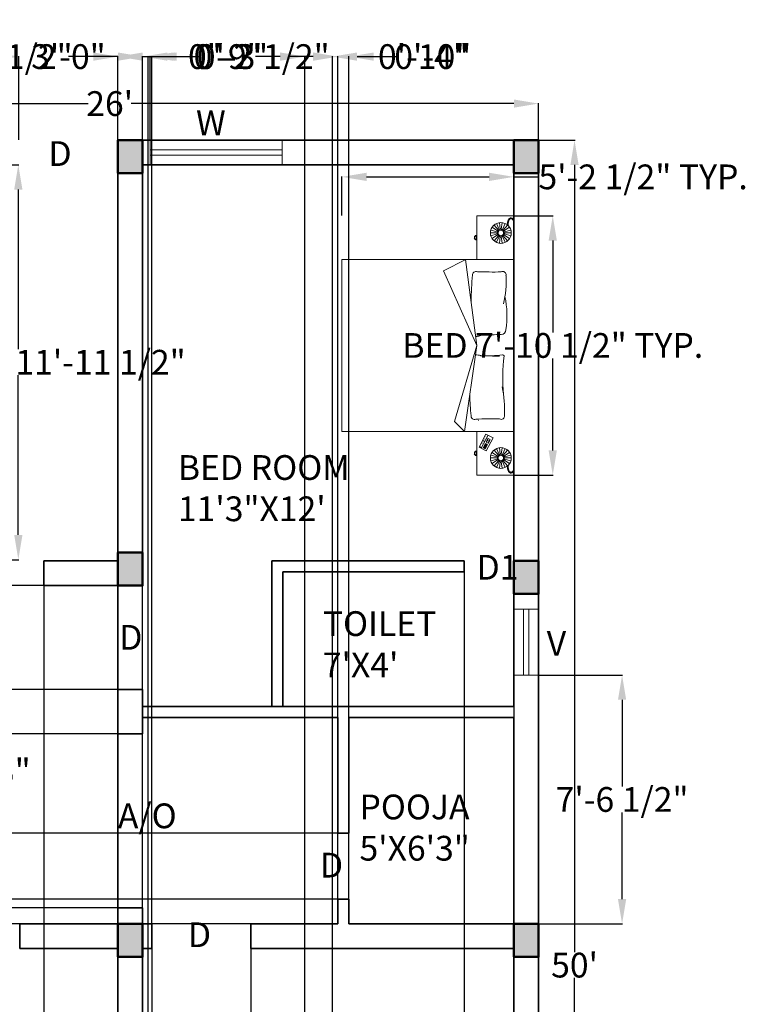
# Model space of a CAD drawing. Units: inches. Extents: x 113 to 575, y 111 to 799.
# Tile 4 of 4: x 301 to 565, y 441 to 799. Entities that reach past the tile are written whole.
import ezdxf

# ---------------------------------------------------------------- set-up
doc = ezdxf.new("R2010")
doc.units = ezdxf.units.IN
doc.header["$MEASUREMENT"] = 0
for name, color, linetype, lineweight in [('A-ANNO-DIMS', 2, 'Continuous', 18), ('A-ANNO-TEXT', 7, 'Continuous', 18), ('A-AREA-IDEN', 7, 'Continuous', 25), ('A-COLS', 7, 'Continuous', 50), ('A-COLS-PATT', 252, 'Continuous', 13), ('A-FURN', 8, 'Continuous', 18), ('A-GLAZ', 4, 'Continuous', 18), ('A-WALL', 7, 'Continuous', 35)]:
    doc.layers.add(name, color=color, linetype=linetype, lineweight=lineweight)
doc.styles.get("Standard").update_dxf_attribs({"font": 'arial.ttf'})
doc.dimstyles.get("Standard").update_dxf_attribs({"dimtxt": 9, "dimasz": 9, "dimexe": 0.18, "dimexo": 0.0625, "dimgap": 0.09, "dimtad": 0, "dimtih": 1, "dimtoh": 1, "dimdec": 0, "dimzin": 0, "dimdsep": 46, "dimlunit": 3, "dimtxsty": 'Standard', "dimcen": 0.09, "dimadec": 0, "dimazin": 0, "dimtfac": 1, "dimtdec": 0, "dimtofl": 0, "dimtmove": 0, "dimatfit": 3, "dimfxl": 1, "dimtolj": 1, "dimtzin": 0, "dimarcsym": 0})

# ---------------------------------------------------------------- blocks, each defined once
blk = doc.blocks.new('23')
for p, q in [((198.051, 218.551), (197.59, 218.551)), ((197.59, 218.551), (197.59, 218.161)), ((198.051, 218.551), (197.59, 218.551)), ((197.688, 218.484), (197.741, 218.439)), ((197.711, 218.505), (197.749, 218.446)), ((197.74, 218.518), (197.76, 218.451)), ((197.771, 218.522), (197.771, 218.452)), ((197.771, 218.522), (197.771, 218.452)), ((197.802, 218.518), (197.782, 218.451)), ((197.792, 218.446), (197.83, 218.505)), ((197.801, 218.439), (197.854, 218.484)), ((198.051, 216.732), (198.051, 218.551)), ((198.051, 218.551), (198.96, 218.551)), ((198.051, 218.551), (199.869, 218.551)), ((198.051, 218.551), (198.051, 218.161)), ((199.869, 218.551), (200.331, 218.551)), ((199.869, 218.551), (200.331, 218.551)), ((199.869, 218.551), (199.869, 216.732)), ((200.12, 218.439), (200.067, 218.484)), ((200.129, 218.446), (200.091, 218.505)), ((200.119, 218.518), (200.139, 218.451)), ((200.15, 218.522), (200.15, 218.452)), ((200.15, 218.522), (200.15, 218.452)), ((200.181, 218.518), (200.161, 218.451)), ((200.209, 218.505), (200.171, 218.446)), ((200.233, 218.484), (200.18, 218.439)), ((200.331, 218.551), (200.331, 218.161)), ((197.662, 218.428), (197.731, 218.418)), ((197.662, 218.397), (197.731, 218.407)), ((197.671, 218.458), (197.735, 218.429)), ((197.671, 218.367), (197.735, 218.396)), ((197.688, 218.341), (197.741, 218.387)), ((197.711, 218.32), (197.749, 218.379)), ((197.742, 218.419), (197.732, 218.423)), ((197.744, 218.425), (197.734, 218.427)), ((197.76, 218.375), (197.74, 218.307)), ((197.765, 218.384), (197.765, 218.373)), ((197.772, 218.383), (197.77, 218.373)), ((197.771, 218.373), (197.771, 218.303)), ((197.771, 218.373), (197.771, 218.303)), ((197.782, 218.375), (197.802, 218.307)), ((197.786, 218.438), (197.795, 218.444)), ((197.792, 218.379), (197.83, 218.32)), ((197.793, 218.431), (197.799, 218.44)), ((197.801, 218.387), (197.854, 218.341)), ((197.807, 218.429), (197.87, 218.458)), ((197.807, 218.396), (197.87, 218.367)), ((197.81, 218.418), (197.879, 218.428)), ((197.81, 218.407), (197.879, 218.397)), ((200.111, 218.418), (200.042, 218.428)), ((200.111, 218.407), (200.042, 218.397)), ((200.114, 218.429), (200.05, 218.458)), ((200.114, 218.396), (200.05, 218.367)), ((200.12, 218.387), (200.067, 218.341)), ((200.129, 218.379), (200.091, 218.32)), ((200.139, 218.375), (200.119, 218.307)), ((200.127, 218.431), (200.122, 218.44)), ((200.134, 218.438), (200.125, 218.444)), ((200.149, 218.383), (200.151, 218.373)), ((200.15, 218.373), (200.15, 218.303)), ((200.15, 218.373), (200.15, 218.303)), ((200.155, 218.384), (200.155, 218.373)), ((200.161, 218.375), (200.181, 218.307)), ((200.209, 218.32), (200.171, 218.379)), ((200.177, 218.425), (200.187, 218.427)), ((200.179, 218.419), (200.188, 218.423)), ((200.233, 218.341), (200.18, 218.387)), ((200.25, 218.458), (200.186, 218.429)), ((200.25, 218.367), (200.186, 218.396)), ((200.259, 218.428), (200.189, 218.418)), ((200.259, 218.397), (200.189, 218.407)), ((199.897, 218.255), (199.936, 218.33)), ((199.909, 218.279), (200.047, 218.206)), ((199.936, 218.33), (200.074, 218.257)), ((199.943, 218.278), (199.955, 218.299)), ((199.961, 218.269), (199.943, 218.278)), ((199.955, 218.299), (199.972, 218.29)), ((199.972, 218.29), (199.961, 218.269)), ((199.966, 218.267), (199.977, 218.288)), ((199.983, 218.257), (199.966, 218.267)), ((199.977, 218.288), (199.994, 218.278)), ((199.994, 218.278), (199.983, 218.257)), ((199.997, 218.25), (200.008, 218.271)), ((200.047, 218.235), (200.002, 218.259)), ((200.048, 218.238), (200.003, 218.262)), ((200.05, 218.241), (200.004, 218.265)), ((200.052, 218.245), (200.007, 218.269)), ((200.053, 218.247), (200.008, 218.271)), ((197.592, 218.158), (198.049, 218.158)), ((197.829, 218.158), (197.812, 218.158)), ((197.812, 218.158), (197.812, 218.151)), ((197.829, 218.151), (197.829, 218.158)), ((198.96, 218.158), (198.051, 218.039)), ((198.171, 217.806), (198.96, 218.158)), ((199.763, 217.922), (198.96, 218.158)), ((198.96, 218.158), (199.869, 218.028)), ((200.329, 218.158), (199.872, 218.158)), ((200.034, 218.183), (199.897, 218.255)), ((200.042, 218.226), (199.997, 218.25)), ((200.044, 218.23), (199.999, 218.254)), ((200.046, 218.233), (200, 218.257)), ((200.074, 218.257), (200.034, 218.183)), ((200.053, 218.247), (200.042, 218.226)), ((200.092, 218.151), (200.092, 218.158)), ((200.092, 218.158), (200.108, 218.158)), ((200.108, 218.158), (200.108, 218.151)), ((197.799, 218.149), (197.799, 218.144)), ((197.84, 218.151), (197.801, 218.151)), ((197.801, 218.141), (197.805, 218.141)), ((197.808, 218.139), (197.808, 218.135)), ((197.81, 218.133), (197.831, 218.133)), ((197.833, 218.135), (197.833, 218.141)), ((197.833, 218.141), (197.84, 218.141)), ((197.842, 218.144), (197.842, 218.149)), ((200.078, 218.144), (200.078, 218.149)), ((200.081, 218.151), (200.12, 218.151)), ((200.087, 218.141), (200.081, 218.141)), ((200.087, 218.135), (200.087, 218.141)), ((200.111, 218.133), (200.09, 218.133)), ((200.113, 218.139), (200.113, 218.135)), ((200.12, 218.141), (200.115, 218.141)), ((200.122, 218.149), (200.122, 218.144)), ((198.051, 218.042), (198.171, 217.806)), ((199.869, 218.028), (199.763, 217.922)), ((198.96, 216.732), (198.051, 216.732)), ((198.96, 216.732), (199.869, 216.732))]:
    blk.add_line(p, q)
for centre, radius in [((197.771, 218.413), 0.11), ((200.15, 218.413), 0.11), ((197.771, 218.413), 0.0397), ((197.771, 218.413), 0.0294), ((200.15, 218.413), 0.0397), ((200.15, 218.413), 0.0294)]:
    blk.add_circle(centre, radius)
for centre, radius, start, end in [((198.213, 218.433), 0.035, 78.7278, 211.6095), ((198.213, 218.433), 0.035, 78.7278, 211.6095), ((198.278, 217.379), 1.09, 77.0564, 93.0488), ((198.278, 217.379), 1.09, 77.0564, 93.0488), ((198.648, 217.496), 0.982, 81.4702, 102.1033), ((198.648, 217.496), 0.982, 81.4702, 102.1033), ((198.794, 218.417), 0.0503, 0, 90), ((198.794, 218.417), 0.0503, 0, 90), ((194.58, 218.326), 3.604, 357.4333, 1.4038), ((194.58, 218.326), 3.604, 357.4333, 1.4038), ((192.856, 218.12), 5.995, 0.9126, 2.8341), ((192.856, 218.12), 5.995, 0.9126, 2.8341), ((199.106, 218.403), 0.0559, 128.2265, 148.4948), ((198.082, 218.271), 0.989, 355.8781, 9.3556), ((205.063, 218.104), 5.995, 177.1659, 179.0874), ((199.31, 220.76), 2.326, 264.0962, 274.1102), ((199.106, 218.403), 0.0559, 41.3461, 41.8512), ((199.642, 217.363), 1.09, 86.9512, 102.9436), ((199.642, 217.363), 1.09, 86.9512, 102.9436), ((199.707, 218.417), 0.035, 328.3905, 101.2722), ((199.707, 218.417), 0.035, 328.3905, 101.2722), ((203.34, 218.31), 3.604, 178.5962, 182.5667), ((203.34, 218.31), 3.604, 178.5962, 182.5667), ((197.592, 218.161), 0.0024, 180, 270), ((198.214, 218.15), 0.0362, 156.1084, 279.6576), ((198.214, 218.15), 0.0362, 156.1084, 279.6576), ((198.785, 218.186), 0.0722, 2.6698, 24.3744), ((198.551, 218.114), 0.317, 5.8626, 18.7589), ((199.2, 218.15), 0.14, 159.1632, 182.3748), ((199.134, 218.17), 0.0722, 155.6256, 177.3302), ((199.755, 218.175), 0.00192, 180, 270), ((199.968, 218.228), 0.00141, 90, 270), ((199.968, 218.228), 0.00141, 270, 90), ((199.972, 218.235), 0.00141, 90, 270), ((199.972, 218.235), 0.00141, 270, 90), ((200.031, 218.191), 0.00141, 90, 270), ((200.031, 218.191), 0.00141, 270, 90), ((200.037, 218.2), 0.00141, 90, 270), ((200.037, 218.2), 0.00141, 270, 90), ((200.329, 218.161), 0.0024, 270, 0), ((197.801, 218.149), 0.0024, 90, 180), ((197.801, 218.144), 0.0024, 180, 270), ((197.805, 218.139), 0.0024, 0, 90), ((197.81, 218.135), 0.0024, 180, 270), ((197.831, 218.135), 0.0024, 270, 0), ((197.84, 218.149), 0.0024, 0, 90), ((197.84, 218.144), 0.0024, 270, 0), ((198.502, 220.904), 2.805, 264.1139, 269.9157), ((198.502, 220.904), 2.805, 264.1139, 269.9157), ((199.418, 220.888), 2.805, 271.2842, 275.8861), ((199.418, 220.888), 2.805, 271.2842, 275.8861), ((199.706, 218.134), 0.0362, 260.3424, 23.8916), ((199.706, 218.134), 0.0362, 260.3424, 23.8916), ((200.081, 218.149), 0.0024, 90, 180), ((200.081, 218.144), 0.0024, 180, 270), ((200.09, 218.135), 0.0024, 180, 270), ((200.111, 218.135), 0.0024, 270, 0), ((200.115, 218.139), 0.0024, 90, 180), ((200.12, 218.149), 0.0024, 0, 90), ((200.12, 218.144), 0.0024, 270, 0)]:
    blk.add_arc(centre, radius, start, end)
for points, knots in [([(197.686, 218.482), (197.674, 218.482), (197.661, 218.483), (197.634, 218.491), (197.617, 218.497), (197.608, 218.527), (197.618, 218.537), (197.629, 218.548), (197.631, 218.549), (197.633, 218.551)], [0.0077183, 0.0077183, 0.0077183, 0.0077183, 0.0428867, 0.0428867, 0.0785443, 0.0785443, 0.1084778, 0.1084778, 0.1132873, 0.1132873, 0.1132873, 0.1132873]), ([(197.694, 218.491), (197.677, 218.49), (197.651, 218.49), (197.607, 218.519), (197.631, 218.539), (197.645, 218.551)], [0, 0, 0, 0, 0.0514038, 0.0806942, 0.123773, 0.123773, 0.123773, 0.123773]), ([(200.227, 218.491), (200.244, 218.49), (200.27, 218.49), (200.314, 218.519), (200.29, 218.539), (200.275, 218.551)], [0, 0, 0, 0, 0.0514038, 0.0806942, 0.123773, 0.123773, 0.123773, 0.123773]), ([(200.235, 218.482), (200.247, 218.482), (200.26, 218.483), (200.287, 218.491), (200.304, 218.497), (200.313, 218.527), (200.303, 218.537), (200.291, 218.548), (200.29, 218.549), (200.288, 218.551)], [0.0077183, 0.0077183, 0.0077183, 0.0077183, 0.0428867, 0.0428867, 0.0785443, 0.0785443, 0.1084778, 0.1084778, 0.1132873, 0.1132873, 0.1132873, 0.1132873])]:
    blk.add_open_spline(points, degree=3, knots=knots)
at = {"width": 3}
blk.add_text('12 00', height=0.0101, rotation=330.6435, dxfattribs=at).set_placement((199.915, 218.257))
blk = doc.blocks.new('*D6')
at = {"layer": 'A-ANNO-DIMS', "color": 0, "lineweight": -2, "transparency": 16777216}
for p, q in [((177.49, 754.88), (177.49, 768.27)), ((186.49, 768.09), (325.69, 768.09)), ((480.49, 768.09), (341.3, 768.09)), ((489.49, 754.88), (489.49, 768.27))]:
    blk.add_line(p, q, dxfattribs=at)
at = {"layer": 'A-ANNO-DIMS', "color": 0, "transparency": 16777216}
for points in [[(186.49, 769.59), (186.49, 766.59), (177.49, 768.09)], [(480.49, 769.59), (480.49, 766.59), (489.49, 768.09)]]:
    blk.add_solid(points, dxfattribs=at)
at = {"layer": 'Defpoints', "color": 0, "transparency": 16777216}
for p in [(489.49, 768.09), (177.49, 754.81), (489.49, 754.81)]:
    blk.add_point(p, dxfattribs=at)
at = {"layer": 'A-ANNO-DIMS', "color": 0, "transparency": 16777216, "insert": (333.49, 768.09), "char_height": 9, "attachment_point": 5}
blk.add_mtext("\\A1;26'", dxfattribs=at)
blk = doc.blocks.new('*D7')
at = {"layer": 'A-ANNO-DIMS', "color": 0, "lineweight": -2, "transparency": 16777216}
for p, q in [((489.56, 754.81), (502.74, 754.81)), ((502.56, 745.81), (502.56, 459.5)), ((502.56, 163.81), (502.56, 450.13)), ((489.56, 154.81), (502.74, 154.81))]:
    blk.add_line(p, q, dxfattribs=at)
at = {"layer": 'A-ANNO-DIMS', "color": 0, "transparency": 16777216}
for points in [[(501.06, 745.81), (504.06, 745.81), (502.56, 754.81)], [(501.06, 163.81), (504.06, 163.81), (502.56, 154.81)]]:
    blk.add_solid(points, dxfattribs=at)
at = {"layer": 'Defpoints', "color": 0, "transparency": 16777216}
for p in [(489.49, 754.81), (489.49, 154.81), (502.56, 154.81)]:
    blk.add_point(p, dxfattribs=at)
at = {"layer": 'A-ANNO-DIMS', "color": 0, "transparency": 16777216, "insert": (502.56, 454.81), "char_height": 9, "attachment_point": 5}
blk.add_mtext("\\A1;50'", dxfattribs=at)
blk = doc.blocks.new('WIN-48IN')
for p, q in [((0, 9), (0, 0)), ((48, 9), (48, 0)), ((0, 5.5), (48, 5.5)), ((0, 3.5), (48, 3.5))]:
    blk.add_line(p, q)
blk = doc.blocks.new('VENT-24IN')
for p, q in [((0, 24), (9, 24)), ((3.5, 0), (3.5, 24)), ((5.5, 0), (5.5, 24)), ((0, 0), (9, 0))]:
    blk.add_line(p, q)
blk = doc.blocks.new('*D14')
at = {"layer": 'A-ANNO-DIMS', "color": 0, "lineweight": -2, "transparency": 16777216}
for p, q in [((480.56, 727.29), (494.82, 727.29)), ((494.64, 718.29), (494.64, 684.88)), ((494.64, 641.99), (494.64, 675.4)), ((480.56, 632.99), (494.82, 632.99))]:
    blk.add_line(p, q, dxfattribs=at)
at = {"layer": 'A-ANNO-DIMS', "color": 0, "transparency": 16777216}
for points in [[(493.14, 718.29), (496.14, 718.29), (494.64, 727.29)], [(493.14, 641.99), (496.14, 641.99), (494.64, 632.99)]]:
    blk.add_solid(points, dxfattribs=at)
at = {"layer": 'Defpoints', "color": 0, "transparency": 16777216}
for p in [(480.49, 727.29), (480.49, 632.99), (494.64, 632.99)]:
    blk.add_point(p, dxfattribs=at)
at = {"layer": 'A-ANNO-DIMS', "color": 0, "transparency": 16777216, "insert": (494.64, 680.14), "char_height": 9, "attachment_point": 5}
blk.add_mtext('\\A1;BED 7\'-10 1/2" TYP.', dxfattribs=at)
blk = doc.blocks.new('*D15')
at = {"layer": 'A-ANNO-DIMS', "color": 0, "lineweight": -2, "transparency": 16777216}
for p, q in [((417.95, 727.35), (417.95, 741.62)), ((426.95, 741.44), (471.49, 741.44)), ((480.49, 727.35), (480.49, 741.62)), ((480.49, 741.44), (489.49, 741.44))]:
    blk.add_line(p, q, dxfattribs=at)
at = {"layer": 'A-ANNO-DIMS', "color": 0, "transparency": 16777216}
for points in [[(426.95, 742.94), (426.95, 739.94), (417.95, 741.44)], [(471.49, 742.94), (471.49, 739.94), (480.49, 741.44)]]:
    blk.add_solid(points, dxfattribs=at)
at = {"layer": 'Defpoints', "color": 0, "transparency": 16777216}
for p in [(480.49, 741.44), (417.95, 727.29), (480.49, 727.29)]:
    blk.add_point(p, dxfattribs=at)
at = {"layer": 'A-ANNO-DIMS', "color": 0, "transparency": 16777216, "insert": (527.5, 741.44), "char_height": 9, "attachment_point": 5}
blk.add_mtext('\\A1;5\'-2 1/2" TYP.', dxfattribs=at)
blk = doc.blocks.new('*D18')
at = {"layer": 'A-ANNO-DIMS', "color": 0, "lineweight": -2, "transparency": 16777216}
for p, q in [((278.8, 745.81), (300.45, 745.81)), ((300.27, 736.81), (300.27, 678.78)), ((300.27, 611.24), (300.27, 669.28)), ((278.8, 602.24), (300.45, 602.24))]:
    blk.add_line(p, q, dxfattribs=at)
at = {"layer": 'A-ANNO-DIMS', "color": 0, "transparency": 16777216}
for points in [[(298.77, 736.81), (301.77, 736.81), (300.27, 745.81)], [(298.77, 611.24), (301.77, 611.24), (300.27, 602.24)]]:
    blk.add_solid(points, dxfattribs=at)
at = {"layer": 'Defpoints', "color": 0, "transparency": 16777216}
for p in [(278.74, 745.81), (300.27, 745.81), (278.74, 602.24)]:
    blk.add_point(p, dxfattribs=at)
at = {"layer": 'A-ANNO-DIMS', "color": 0, "transparency": 16777216, "insert": (300.27, 674.03), "char_height": 9, "attachment_point": 5}
blk.add_mtext('\\A1;COUNTER 11\'-11 1/2"', dxfattribs=at)
blk = doc.blocks.new('*D26')
at = {"layer": 'A-ANNO-DIMS', "color": 0, "lineweight": -2, "transparency": 16777216}
for p, q in [((395.49, 785.17), (386.49, 785.17)), ((404.49, 241.88), (404.49, 785.35)), ((414.49, 241.88), (414.49, 785.35)), ((423.49, 785.17), (432.49, 785.17))]:
    blk.add_line(p, q, dxfattribs=at)
at = {"layer": 'A-ANNO-DIMS', "color": 0, "transparency": 16777216}
for points in [[(395.49, 786.67), (395.49, 783.67), (404.49, 785.17)], [(423.49, 786.67), (423.49, 783.67), (414.49, 785.17)]]:
    blk.add_solid(points, dxfattribs=at)
at = {"layer": 'Defpoints', "color": 0, "transparency": 16777216}
for p in [(414.49, 785.17), (404.49, 241.81), (414.49, 241.81)]:
    blk.add_point(p, dxfattribs=at)
at = {"layer": 'A-ANNO-DIMS', "color": 0, "transparency": 16777216, "insert": (448.04, 785.17), "char_height": 9, "attachment_point": 5}
blk.add_mtext('\\A1;0\'-10"', dxfattribs=at)
blk = doc.blocks.new('*D27')
at = {"layer": 'A-ANNO-DIMS', "color": 0, "lineweight": -2, "transparency": 16777216}
for p, q in [((327.49, 785.17), (318.49, 785.17)), ((336.49, 202.88), (336.49, 785.35)), ((345.49, 202.88), (345.49, 785.35)), ((354.49, 785.17), (363.49, 785.17))]:
    blk.add_line(p, q, dxfattribs=at)
at = {"layer": 'A-ANNO-DIMS', "color": 0, "transparency": 16777216}
for points in [[(327.49, 786.67), (327.49, 783.67), (336.49, 785.17)], [(354.49, 786.67), (354.49, 783.67), (345.49, 785.17)]]:
    blk.add_solid(points, dxfattribs=at)
at = {"layer": 'Defpoints', "color": 0, "transparency": 16777216}
for p in [(345.49, 785.17), (336.49, 202.81), (345.49, 202.81)]:
    blk.add_point(p, dxfattribs=at)
at = {"layer": 'A-ANNO-DIMS', "color": 0, "transparency": 16777216, "insert": (375.55, 785.17), "char_height": 9, "attachment_point": 5}
blk.add_mtext('\\A1;0\'-9"', dxfattribs=at)
blk = doc.blocks.new('*D29')
at = {"layer": 'A-ANNO-DIMS', "color": 0, "lineweight": -2, "transparency": 16777216}
for p, q in [((291.494828, 785.172567), (282.494828, 785.172567)), ((300.494828, 754.875317), (300.494828, 785.352567)), ((336.494828, 754.875317), (336.494828, 785.352567)), ((345.494828, 785.172567), (354.494828, 785.172567))]:
    blk.add_line(p, q, dxfattribs=at)
at = {"layer": 'A-ANNO-DIMS', "color": 0, "transparency": 16777216}
for points in [[(291.494828, 786.672567), (291.494828, 783.672567), (300.494828, 785.172567)], [(345.494828, 786.672567), (345.494828, 783.672567), (336.494828, 785.172567)]]:
    blk.add_solid(points, dxfattribs=at)
at = {"layer": 'Defpoints', "color": 0, "transparency": 16777216}
for p in [(336.494828, 785.172567), (300.494828, 754.812817), (336.494828, 754.812817)]:
    blk.add_point(p, dxfattribs=at)
at = {"layer": 'A-ANNO-DIMS', "color": 0, "transparency": 16777216, "insert": (318.494828, 785.172567), "char_height": 9, "attachment_point": 5}
blk.add_mtext('\\A1;3\'-0"', dxfattribs=at)
blk = doc.blocks.new('*D31')
at = {"layer": 'A-ANNO-DIMS', "color": 0, "lineweight": -2, "transparency": 16777216}
for p, q in [((147.14, 502.81), (147.14, 511.81)), ((147.14, 511.81), (156.14, 511.81)), ((416.43, 502.81), (146.96, 502.81)), ((147.14, 487.81), (147.14, 493.81)), ((416.43, 478.81), (146.96, 478.81))]:
    blk.add_line(p, q, dxfattribs=at)
at = {"layer": 'A-ANNO-DIMS', "color": 0, "transparency": 16777216}
for points in [[(145.64, 493.81), (148.64, 493.81), (147.14, 502.81)], [(145.64, 487.81), (148.64, 487.81), (147.14, 478.81)]]:
    blk.add_solid(points, dxfattribs=at)
at = {"layer": 'Defpoints', "color": 0, "transparency": 16777216}
for p in [(147.14, 502.81), (416.49, 502.81), (416.49, 478.81)]:
    blk.add_point(p, dxfattribs=at)
at = {"layer": 'A-ANNO-DIMS', "color": 0, "transparency": 16777216, "insert": (168.26, 511.81), "char_height": 9, "attachment_point": 5}
blk.add_mtext('\\A1;2\'-0"', dxfattribs=at)
blk = doc.blocks.new('*D32')
at = {"layer": 'A-ANNO-DIMS', "color": 0, "lineweight": -2, "transparency": 16777216}
for p, q in [((480.49, 601.75), (480.49, 124.27)), ((462.45, 597.75), (462.45, 124.27)), ((453.45, 124.45), (444.45, 124.45)), ((489.49, 124.45), (498.49, 124.45))]:
    blk.add_line(p, q, dxfattribs=at)
at = {"layer": 'A-ANNO-DIMS', "color": 0, "transparency": 16777216}
for points in [[(453.45, 125.95), (453.45, 122.95), (462.45, 124.45)], [(489.49, 125.95), (489.49, 122.95), (480.49, 124.45)]]:
    blk.add_solid(points, dxfattribs=at)
at = {"layer": 'Defpoints', "color": 0, "transparency": 16777216}
for p in [(480.49, 601.81), (462.45, 597.81), (480.49, 124.45)]:
    blk.add_point(p, dxfattribs=at)
at = {"layer": 'A-ANNO-DIMS', "color": 0, "transparency": 16777216, "insert": (510.12, 124.45), "char_height": 9, "attachment_point": 5}
blk.add_mtext('\\A1;1\'-6"', dxfattribs=at)
blk = doc.blocks.new('*D40')
at = {"layer": 'A-ANNO-DIMS', "color": 0, "lineweight": -2, "transparency": 16777216}
for p, q in [((489.56, 560.29), (520.03, 560.29)), ((519.85, 551.29), (519.85, 519.79)), ((519.85, 478.81), (519.85, 510.31)), ((489.56, 469.81), (520.03, 469.81))]:
    blk.add_line(p, q, dxfattribs=at)
at = {"layer": 'A-ANNO-DIMS', "color": 0, "transparency": 16777216}
for points in [[(518.35, 551.29), (521.35, 551.29), (519.85, 560.29)], [(518.35, 478.81), (521.35, 478.81), (519.85, 469.81)]]:
    blk.add_solid(points, dxfattribs=at)
at = {"layer": 'Defpoints', "color": 0, "transparency": 16777216}
for p in [(489.49, 560.29), (489.49, 469.81), (519.85, 469.81)]:
    blk.add_point(p, dxfattribs=at)
at = {"layer": 'A-ANNO-DIMS', "color": 0, "transparency": 16777216, "insert": (519.85, 515.05), "char_height": 9, "attachment_point": 5}
blk.add_mtext('\\A1;7\'-6 1/2"', dxfattribs=at)
blk = doc.blocks.new('*D41')
at = {"layer": 'A-ANNO-DIMS', "color": 0, "lineweight": -2, "transparency": 16777216}
for p, q in [((407.49, 785.17), (398.49, 785.17)), ((416.49, 469.88), (416.49, 785.35)), ((420.49, 469.88), (420.49, 785.35)), ((429.49, 785.17), (438.49, 785.17))]:
    blk.add_line(p, q, dxfattribs=at)
at = {"layer": 'A-ANNO-DIMS', "color": 0, "transparency": 16777216}
for points in [[(407.49, 786.67), (407.49, 783.67), (416.49, 785.17)], [(429.49, 786.67), (429.49, 783.67), (420.49, 785.17)]]:
    blk.add_solid(points, dxfattribs=at)
at = {"layer": 'Defpoints', "color": 0, "transparency": 16777216}
for p in [(420.49, 785.17), (416.49, 469.81), (420.49, 469.81)]:
    blk.add_point(p, dxfattribs=at)
at = {"layer": 'A-ANNO-DIMS', "color": 0, "transparency": 16777216, "insert": (450.55, 785.17), "char_height": 9, "attachment_point": 5}
blk.add_mtext('\\A1;0\'-4"', dxfattribs=at)
blk = doc.blocks.new('*D42')
at = {"layer": 'A-ANNO-DIMS', "color": 0, "lineweight": -2, "transparency": 16777216}
for p, q in [((327.49, 785.17), (318.49, 785.17)), ((336.49, 754.88), (336.49, 785.35)), ((348.21, 754.88), (348.21, 785.35)), ((357.21, 785.17), (366.21, 785.17))]:
    blk.add_line(p, q, dxfattribs=at)
at = {"layer": 'A-ANNO-DIMS', "color": 0, "transparency": 16777216}
for points in [[(327.49, 786.67), (327.49, 783.67), (336.49, 785.17)], [(357.21, 786.67), (357.21, 783.67), (348.21, 785.17)]]:
    blk.add_solid(points, dxfattribs=at)
at = {"layer": 'Defpoints', "color": 0, "transparency": 16777216}
for p in [(336.49, 785.17), (336.49, 754.81), (348.21, 754.81)]:
    blk.add_point(p, dxfattribs=at)
at = {"layer": 'A-ANNO-DIMS', "color": 0, "transparency": 16777216, "insert": (292.46, 785.17), "char_height": 9, "attachment_point": 5}
blk.add_mtext('\\A1;0\'-11 1/2"', dxfattribs=at)
blk = doc.blocks.new('*D43')
at = {"layer": 'A-ANNO-DIMS', "color": 0, "lineweight": -2, "transparency": 16777216}
for p, q in [((336.49, 785.17), (327.49, 785.17)), ((345.49, 241.88), (345.49, 785.35)), ((347.52, 241.88), (347.52, 785.35)), ((356.52, 785.17), (365.52, 785.17))]:
    blk.add_line(p, q, dxfattribs=at)
at = {"layer": 'A-ANNO-DIMS', "color": 0, "transparency": 16777216}
for points in [[(336.49, 786.67), (336.49, 783.67), (345.49, 785.17)], [(356.52, 786.67), (356.52, 783.67), (347.52, 785.17)]]:
    blk.add_solid(points, dxfattribs=at)
at = {"layer": 'Defpoints', "color": 0, "transparency": 16777216}
for p in [(347.52, 785.17), (345.49, 241.81), (347.52, 241.81)]:
    blk.add_point(p, dxfattribs=at)
at = {"layer": 'A-ANNO-DIMS', "color": 0, "transparency": 16777216, "insert": (377.57, 785.17), "char_height": 9, "attachment_point": 5}
blk.add_mtext('\\A1;0\'-2"', dxfattribs=at)
blk = doc.blocks.new('*D45')
at = {"layer": 'A-ANNO-DIMS', "color": 0, "lineweight": -2, "transparency": 16777216}
for p, q in [((336.43, 592.81), (146.96, 592.81)), ((147.14, 583.81), (147.14, 578.61)), ((147.14, 564.04), (147.14, 569.24)), ((336.43, 555.04), (146.96, 555.04))]:
    blk.add_line(p, q, dxfattribs=at)
at = {"layer": 'A-ANNO-DIMS', "color": 0, "transparency": 16777216}
for points in [[(145.64, 583.81), (148.64, 583.81), (147.14, 592.81)], [(145.64, 564.04), (148.64, 564.04), (147.14, 555.04)]]:
    blk.add_solid(points, dxfattribs=at)
at = {"layer": 'Defpoints', "color": 0, "transparency": 16777216}
for p in [(147.14, 592.81), (336.49, 592.81), (336.49, 555.04)]:
    blk.add_point(p, dxfattribs=at)
at = {"layer": 'A-ANNO-DIMS', "color": 0, "transparency": 16777216, "insert": (147.14, 573.93), "char_height": 9, "attachment_point": 5}
blk.add_mtext('\\A1;3\'-2"', dxfattribs=at)
blk = doc.blocks.new('*D46')
at = {"layer": 'A-ANNO-DIMS', "color": 0, "lineweight": -2, "transparency": 16777216}
for p, q in [((336.43, 538.91), (146.96, 538.91)), ((147.14, 529.91), (147.14, 512.01)), ((147.14, 484.62), (147.14, 502.52)), ((336.43, 475.62), (146.96, 475.62))]:
    blk.add_line(p, q, dxfattribs=at)
at = {"layer": 'A-ANNO-DIMS', "color": 0, "transparency": 16777216}
for points in [[(145.64, 529.91), (148.64, 529.91), (147.14, 538.91)], [(145.64, 484.62), (148.64, 484.62), (147.14, 475.62)]]:
    blk.add_solid(points, dxfattribs=at)
at = {"layer": 'Defpoints', "color": 0, "transparency": 16777216}
for p in [(147.14, 538.91), (336.49, 538.91), (336.49, 475.62)]:
    blk.add_point(p, dxfattribs=at)
at = {"layer": 'A-ANNO-DIMS', "color": 0, "transparency": 16777216, "insert": (147.14, 507.27), "char_height": 9, "attachment_point": 5}
blk.add_mtext('\\A1;5\'-3 1/2"', dxfattribs=at)
blk = doc.blocks.new('*D47')
at = {"layer": 'A-ANNO-DIMS', "color": 0, "lineweight": -2, "transparency": 16777216}
for p, q in [((348.815003, 460.750317), (348.815003, 124.273067)), ((384.815003, 460.750317), (384.815003, 124.273067)), ((339.815003, 124.453067), (330.815003, 124.453067)), ((393.815003, 124.453067), (402.815003, 124.453067))]:
    blk.add_line(p, q, dxfattribs=at)
at = {"layer": 'A-ANNO-DIMS', "color": 0, "transparency": 16777216}
for points in [[(339.815003, 125.953067), (339.815003, 122.953067), (348.815003, 124.453067)], [(393.815003, 125.953067), (393.815003, 122.953067), (384.815003, 124.453067)]]:
    blk.add_solid(points, dxfattribs=at)
at = {"layer": 'Defpoints', "color": 0, "transparency": 16777216}
for p in [(348.815003, 460.812817), (384.815003, 460.812817), (384.815003, 124.453067)]:
    blk.add_point(p, dxfattribs=at)
at = {"layer": 'A-ANNO-DIMS', "color": 0, "transparency": 16777216, "insert": (366.815003, 124.453067), "char_height": 9, "attachment_point": 5}
blk.add_mtext('\\A1;3\'-0"', dxfattribs=at)
blk = doc.blocks.new('*D49')
at = {"layer": 'A-ANNO-DIMS', "color": 0, "lineweight": -2, "transparency": 16777216}
for p, q in [((309.494828, 592.750317), (309.494828, 124.273067)), ((336.494828, 592.750317), (336.494828, 124.273067)), ((300.494828, 124.453067), (291.494828, 124.453067)), ((345.494828, 124.453067), (354.494828, 124.453067))]:
    blk.add_line(p, q, dxfattribs=at)
at = {"layer": 'A-ANNO-DIMS', "color": 0, "transparency": 16777216}
for points in [[(300.494828, 125.953067), (300.494828, 122.953067), (309.494828, 124.453067)], [(345.494828, 125.953067), (345.494828, 122.953067), (336.494828, 124.453067)]]:
    blk.add_solid(points, dxfattribs=at)
at = {"layer": 'Defpoints', "color": 0, "transparency": 16777216}
for p in [(309.494828, 592.812817), (336.494828, 592.812817), (336.494828, 124.453067)]:
    blk.add_point(p, dxfattribs=at)
at = {"layer": 'A-ANNO-DIMS', "color": 0, "transparency": 16777216, "insert": (322.994828, 124.453067), "char_height": 9, "attachment_point": 5}
blk.add_mtext('\\A1;2\'-3"', dxfattribs=at)
blk = doc.blocks.new('*D54')
at = {"layer": 'A-ANNO-DIMS', "color": 0, "lineweight": -2, "transparency": 16777216}
for p, q in [((147.14, 487.81), (147.14, 496.81)), ((147.14, 496.81), (156.14, 496.81)), ((416.43, 478.81), (146.96, 478.81)), ((416.43, 469.81), (146.96, 469.81)), ((147.14, 460.81), (147.14, 451.81))]:
    blk.add_line(p, q, dxfattribs=at)
at = {"layer": 'A-ANNO-DIMS', "color": 0, "transparency": 16777216}
for points in [[(145.64, 487.81), (148.64, 487.81), (147.14, 478.81)], [(145.64, 460.81), (148.64, 460.81), (147.14, 469.81)]]:
    blk.add_solid(points, dxfattribs=at)
at = {"layer": 'Defpoints', "color": 0, "transparency": 16777216}
for p in [(147.14, 478.81), (416.49, 478.81), (416.49, 469.81)]:
    blk.add_point(p, dxfattribs=at)
at = {"layer": 'A-ANNO-DIMS', "color": 0, "transparency": 16777216, "insert": (168.19, 496.81), "char_height": 9, "attachment_point": 5}
blk.add_mtext('\\A1;0\'-9"', dxfattribs=at)
blk = doc.blocks.new('*D55')
at = {"layer": 'A-ANNO-DIMS', "color": 0, "lineweight": -2, "transparency": 16777216}
for p, q in [((336.49, 785.17), (327.49, 785.17)), ((345.49, 475.68), (345.49, 785.35)), ((348.82, 469.88), (348.82, 785.35)), ((357.82, 785.17), (366.82, 785.17))]:
    blk.add_line(p, q, dxfattribs=at)
at = {"layer": 'A-ANNO-DIMS', "color": 0, "transparency": 16777216}
for points in [[(336.49, 786.67), (336.49, 783.67), (345.49, 785.17)], [(357.82, 786.67), (357.82, 783.67), (348.82, 785.17)]]:
    blk.add_solid(points, dxfattribs=at)
at = {"layer": 'Defpoints', "color": 0, "transparency": 16777216}
for p in [(348.82, 785.17), (345.49, 475.62), (348.82, 469.81)]:
    blk.add_point(p, dxfattribs=at)
at = {"layer": 'A-ANNO-DIMS', "color": 0, "transparency": 16777216, "insert": (389.35, 785.17), "char_height": 9, "attachment_point": 5}
blk.add_mtext('\\A1;0\'-3 1/2"', dxfattribs=at)
blk = doc.blocks.new('*D56')
at = {"layer": 'A-ANNO-DIMS', "color": 0, "lineweight": -2, "transparency": 16777216}
for p, q in [((147.14, 484.62), (147.14, 493.62)), ((147.14, 493.62), (156.14, 493.62)), ((336.43, 475.62), (146.96, 475.62)), ((336.43, 469.81), (146.96, 469.81)), ((147.14, 460.81), (147.14, 451.81))]:
    blk.add_line(p, q, dxfattribs=at)
at = {"layer": 'A-ANNO-DIMS', "color": 0, "transparency": 16777216}
for points in [[(145.64, 484.62), (148.64, 484.62), (147.14, 475.62)], [(145.64, 460.81), (148.64, 460.81), (147.14, 469.81)]]:
    blk.add_solid(points, dxfattribs=at)
at = {"layer": 'Defpoints', "color": 0, "transparency": 16777216}
for p in [(147.14, 475.62), (336.49, 475.62), (336.49, 469.81)]:
    blk.add_point(p, dxfattribs=at)
at = {"layer": 'A-ANNO-DIMS', "color": 0, "transparency": 16777216, "insert": (168.19, 493.62), "char_height": 9, "attachment_point": 5}
blk.add_mtext('\\A1;0\'-6"', dxfattribs=at)

msp = doc.modelspace()

# ---------------------------------------------------------------- hatches: boundary and pattern name
at = {"layer": 'A-COLS-PATT'}
h = msp.add_hatch(color=256, dxfattribs=at)
h.dxf.hatch_style = 1
h.paths.add_polyline_path([(186.49, 754.81), (177.49, 754.81), (177.49, 742.81), (186.49, 742.81)])
h.paths.add_polyline_path([(345.49, 754.81), (336.49, 754.81), (336.49, 742.81), (345.49, 742.81)])
h.paths.add_polyline_path([(489.49, 754.81), (480.49, 754.81), (480.49, 742.81), (489.49, 742.81)])
h.paths.add_polyline_path([(489.49, 601.81), (480.49, 601.81), (480.49, 589.81), (489.49, 589.81)])
h.paths.add_polyline_path([(345.49, 604.81), (336.49, 604.81), (336.49, 592.81), (345.49, 592.81)])
h.paths.add_polyline_path([(186.49, 604.81), (177.49, 604.81), (177.49, 592.81), (186.49, 592.81)])
h.paths.add_polyline_path([(186.49, 472.81), (177.49, 472.81), (177.49, 460.81), (186.49, 460.81)])
h.paths.add_polyline_path([(345.49, 469.81), (336.49, 469.81), (336.49, 457.81), (345.49, 457.81)])
h.paths.add_polyline_path([(489.49, 469.81), (480.49, 469.81), (480.49, 457.81), (489.49, 457.81)])
h.paths.add_polyline_path([(186.49, 253.81), (177.49, 253.81), (177.49, 241.81), (186.49, 241.81)])
h.paths.add_polyline_path([(345.49, 253.81), (336.49, 253.81), (336.49, 241.81), (345.49, 241.81)])
h.paths.add_polyline_path([(489.49, 253.81), (480.49, 253.81), (480.49, 241.81), (489.49, 241.81)])
h.paths.add_polyline_path([(489.49, 163.81), (477.49, 163.81), (477.49, 154.81), (489.49, 154.81)])
h.paths.add_polyline_path([(348.49, 163.81), (336.49, 163.81), (336.49, 154.81), (348.49, 154.81)])
h.paths.add_polyline_path([(189.49, 163.81), (177.49, 163.81), (177.49, 154.81), (189.49, 154.81)])

# ---------------------------------------------------------------- linework, layer by layer
at = {"layer": 'A-COLS'}
for points in [[(336.49, 754.81), (345.49, 754.81), (345.49, 742.81), (336.49, 742.81)], [(480.49, 754.81), (489.49, 754.81), (489.49, 742.81), (480.49, 742.81)], [(336.49, 604.81), (345.49, 604.81), (345.49, 592.81), (336.49, 592.81)], [(480.49, 601.81), (489.49, 601.81), (489.49, 589.81), (480.49, 589.81)], [(336.49, 469.81), (345.49, 469.81), (345.49, 457.81), (336.49, 457.81)], [(480.49, 469.81), (489.49, 469.81), (489.49, 457.81), (480.49, 457.81)]]:
    msp.add_lwpolyline(points, close=True, dxfattribs=at)
at = {"layer": 'A-WALL'}
for p, q in [((336.49, 592.81), (336.49, 754.81)), ((336.49, 754.81), (489.49, 754.81)), ((489.49, 754.81), (489.49, 154.81)), ((345.49, 745.81), (345.49, 592.81)), ((345.49, 745.81), (480.49, 745.81)), ((480.49, 745.81), (480.49, 548.81)), ((309.49, 601.81), (309.49, 592.81)), ((309.49, 601.81), (336.49, 601.81)), ((392.49, 601.81), (462.45, 601.81)), ((392.49, 601.81), (392.49, 548.81)), ((462.45, 601.81), (462.45, 597.81)), ((396.49, 597.81), (462.45, 597.81)), ((396.49, 597.81), (396.49, 548.81)), ((309.49, 592.81), (345.49, 592.81)), ((336.49, 555.04), (345.49, 555.04)), ((336.49, 538.91), (336.49, 555.04)), ((345.49, 555.04), (345.49, 538.91)), ((345.49, 548.81), (480.49, 548.81)), ((345.49, 544.81), (416.49, 544.81)), ((416.49, 544.81), (416.49, 502.81)), ((420.49, 544.81), (420.49, 502.81)), ((420.49, 544.81), (480.49, 544.81)), ((480.49, 544.81), (480.49, 302.81)), ((336.49, 538.91), (345.49, 538.91)), ((416.49, 502.81), (420.49, 502.81)), ((416.49, 478.81), (420.49, 478.81)), ((416.49, 478.81), (416.49, 469.81)), ((420.49, 478.81), (420.49, 469.81)), ((336.49, 475.62), (345.49, 475.62)), ((336.49, 241.81), (336.49, 475.62)), ((345.49, 475.62), (345.49, 241.81)), ((300.77, 469.81), (300.77, 460.81)), ((300.77, 469.81), (348.82, 469.81)), ((348.82, 469.81), (348.82, 460.81)), ((384.82, 469.81), (384.82, 460.81)), ((384.82, 469.81), (416.49, 469.81)), ((420.49, 469.81), (480.49, 469.81)), ((300.77, 460.81), (336.49, 460.81)), ((345.49, 460.81), (348.82, 460.81)), ((384.82, 460.81), (480.49, 460.81))]:
    msp.add_line(p, q, dxfattribs=at)

# ---------------------------------------------------------------- block references
at = {"layer": 'A-FURN', "xscale": 34.39932596969199, "yscale": 34.39932596969199, "zscale": 34.39932596969199, "rotation": 270}
msp.add_blockref('23', (-7037.5, 7524.24), dxfattribs=at)
at = {"layer": 'A-GLAZ'}
for name, p in [('WIN-48IN', (348.21, 745.81)), ('VENT-24IN', (480.49, 560.29))]:
    msp.add_blockref(name, p, dxfattribs=at)

# ---------------------------------------------------------------- texts
at = {"layer": 'A-ANNO-TEXT', "char_height": 9, "attachment_point": 1}
for s, heights, insert in [('W', [0], (364.91, 765.58)), ('D', [0], (311.21, 754.4)), ('D1', [0], (466.92, 603.98)), ('D', [0], (336.97, 578.5)), ('V', [9], (492.45, 576.28)), ('A/O', [0], (336.48, 513.59)), ('D', [0], (409.94, 495.66)), ('D', [0], (361.91, 470.35))]:
    msp.add_mtext_dynamic_manual_height_columns(s, width=17.4228, gutter_width=1, heights=heights, dxfattribs=dict(at, insert=insert))
at = {"layer": 'A-AREA-IDEN', "char_height": 9, "attachment_point": 1}
for s, insert in [('BED ROOM\\P11\'3"X12\'', (358.3, 640.25)), ("TOILET\\P7'X4'", (411.01, 583.49)), ('DINING\\P12\'6"X10\'3"', (238.38, 544.87)), ('POOJA\\P5\'X6\'3"', (424.34, 516.82))]:
    msp.add_mtext_dynamic_manual_height_columns(s, width=130.397, gutter_width=1, heights=[0], dxfattribs=dict(at, insert=insert))

# ---------------------------------------------------------------- dimensions: what is measured, and where the dimension line sits
at = {"layer": 'A-ANNO-DIMS'}
for base, p1, p2, override, picture, middle in [((336.49, 785.17), (348.21, 754.81), (336.49, 754.81), {"dimdec": 1, "dimlfac": 1, "dimrnd": 0, "dimzin": 1, "dimdsep": 46, "dimlunit": 4, "dimfrac": 2}, '*D42', (292.46, 785.17)), ((348.82, 785.17), (345.49, 475.62), (348.82, 469.81), {"dimdec": 1, "dimlfac": 1, "dimrnd": 0, "dimzin": 1, "dimdsep": 46, "dimlunit": 4, "dimfrac": 2}, '*D55', (389.35, 785.17)), ((336.49, 785.17), (300.49, 754.81), (336.49, 754.81), {"dimdec": 1, "dimlfac": 1, "dimrnd": 0, "dimzin": 1, "dimdsep": 46, "dimlunit": 4, "dimfrac": 2}, '*D29', (318.49, 785.17)), ((345.49, 785.17), (336.49, 202.81), (345.49, 202.81), {"dimdec": 1, "dimlfac": 1, "dimrnd": 0, "dimzin": 1, "dimdsep": 46, "dimlunit": 4, "dimfrac": 2}, '*D27', (375.55, 785.17)), ((347.52, 785.17), (345.49, 241.81), (347.52, 241.81), {"dimdec": 1, "dimlfac": 1, "dimrnd": 0, "dimzin": 1, "dimdsep": 46, "dimlunit": 4, "dimfrac": 2}, '*D43', (377.57, 785.17)), ((414.49, 785.17), (404.49, 241.81), (414.49, 241.81), {"dimdec": 1, "dimlfac": 1, "dimrnd": 0, "dimzin": 1, "dimdsep": 46, "dimlunit": 4, "dimfrac": 2}, '*D26', (448.04, 785.17)), ((420.49, 785.17), (416.49, 469.81), (420.49, 469.81), {"dimdec": 1, "dimlfac": 1, "dimrnd": 0, "dimzin": 1, "dimdsep": 46, "dimlunit": 4, "dimfrac": 2}, '*D41', (450.55, 785.17)), ((489.49, 768.09), (177.49, 754.81), (489.49, 754.81), {"dimclrd": 0, "dimclre": 0, "dimclrt": 0}, '*D6', (333.49, 768.09)), ((480.49, 124.45), (462.45, 597.81), (480.49, 601.81), {"dimdec": 1, "dimlfac": 1, "dimrnd": 0, "dimzin": 1, "dimdsep": 46, "dimlunit": 4, "dimfrac": 2}, '*D32', (510.12, 124.45)), ((336.49, 124.45), (309.49, 592.81), (336.49, 592.81), {"dimdec": 1, "dimlfac": 1, "dimrnd": 0, "dimzin": 1, "dimdsep": 46, "dimlunit": 4, "dimfrac": 2}, '*D49', (322.99, 124.45)), ((384.82, 124.45), (348.82, 460.81), (384.82, 460.81), {"dimdec": 1, "dimlfac": 1, "dimrnd": 0, "dimzin": 1, "dimdsep": 46, "dimlunit": 4, "dimfrac": 2}, '*D47', (366.82, 124.45))]:
    dim = msp.add_linear_dim(base=base, p1=p1, p2=p2, dimstyle='Standard', override=override, dxfattribs=at)
    dim.commit()
    dim.dimension.update_dxf_attribs({"geometry": picture, "text_midpoint": middle})
dim = msp.add_linear_dim(base=(480.49, 741.44), p1=(417.95, 727.29), p2=(480.49, 727.29), text='<> TYP.', dimstyle='Standard', override={"dimdec": 1, "dimlfac": 1, "dimrnd": 0, "dimzin": 1, "dimdsep": 46, "dimlunit": 4, "dimfrac": 2}, dxfattribs=at)
dim.commit()
dim.dimension.update_dxf_attribs({"geometry": '*D15', "text_midpoint": (527.5, 741.44)})
for base, p1, p2, override, picture, middle in [((502.56, 154.81), (489.49, 754.81), (489.49, 154.81), {"dimclrd": 0, "dimclre": 0, "dimclrt": 0}, '*D7', (502.56, 454.81)), ((147.14, 592.81), (336.49, 555.04), (336.49, 592.81), {"dimdec": 1, "dimlfac": 1, "dimrnd": 0, "dimzin": 1, "dimdsep": 46, "dimlunit": 4, "dimfrac": 2}, '*D45', (147.14, 573.93)), ((519.85, 469.81), (489.49, 560.29), (489.49, 469.81), {"dimdec": 1, "dimlfac": 1, "dimrnd": 0, "dimzin": 1, "dimdsep": 46, "dimlunit": 4, "dimfrac": 2}, '*D40', (519.85, 515.05)), ((147.14, 538.91), (336.49, 475.62), (336.49, 538.91), {"dimdec": 1, "dimlfac": 1, "dimrnd": 0, "dimzin": 1, "dimdsep": 46, "dimlunit": 4, "dimfrac": 2}, '*D46', (147.14, 507.27)), ((147.14, 502.81), (416.49, 478.81), (416.49, 502.81), {"dimdec": 1, "dimlfac": 1, "dimrnd": 0, "dimzin": 1, "dimdsep": 46, "dimlunit": 4, "dimfrac": 2}, '*D31', (168.26, 511.81)), ((147.14, 478.81), (416.49, 469.81), (416.49, 478.81), {"dimdec": 1, "dimlfac": 1, "dimrnd": 0, "dimzin": 1, "dimdsep": 46, "dimlunit": 4, "dimfrac": 2}, '*D54', (168.19, 496.81)), ((147.14, 475.62), (336.49, 469.81), (336.49, 475.62), {"dimdec": 1, "dimlfac": 1, "dimrnd": 0, "dimzin": 1, "dimdsep": 46, "dimlunit": 4, "dimfrac": 2}, '*D56', (168.19, 493.62))]:
    dim = msp.add_linear_dim(base=base, p1=p1, p2=p2, angle=90, dimstyle='Standard', override=override, dxfattribs=at)
    dim.commit()
    dim.dimension.update_dxf_attribs({"geometry": picture, "text_midpoint": middle})
for base, p1, p2, angle, text, picture, middle in [((300.27, 745.81), (278.74, 602.24), (278.74, 745.81), 90, 'COUNTER <>', '*D18', (300.27, 674.03)), ((494.64, 632.99), (480.49, 727.29), (480.49, 632.99), 270, 'BED <> TYP.', '*D14', (494.64, 680.14))]:
    dim = msp.add_linear_dim(base=base, p1=p1, p2=p2, angle=angle, text=text, dimstyle='Standard', override={"dimdec": 1, "dimlfac": 1, "dimrnd": 0, "dimzin": 1, "dimdsep": 46, "dimlunit": 4, "dimfrac": 2}, dxfattribs=at)
    dim.commit()
    dim.dimension.update_dxf_attribs({"geometry": picture, "text_midpoint": middle})

doc.saveas('drawing.dxf')
